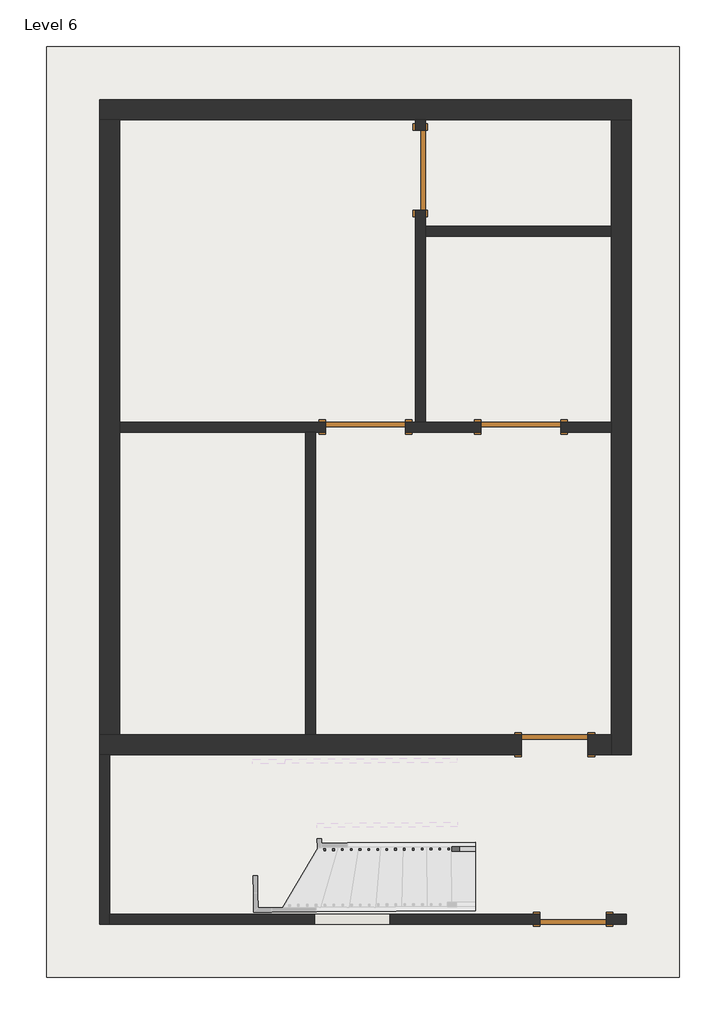
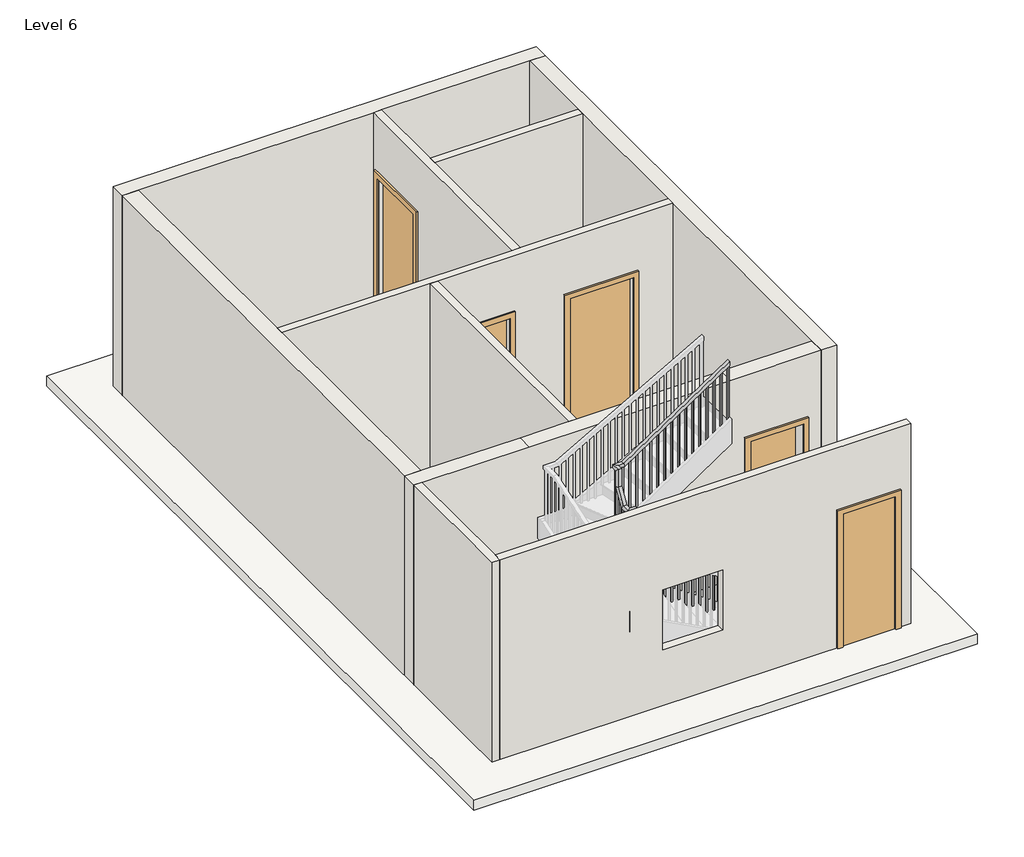
# One storey, part 1 of 2: 10 walls, 5 doors, 1 railing, 1 roof.
"""IFC4 building model written with IfcOpenShell, lengths in millimetres."""

from ifc_helpers import new_model, si_unit, frame, origin, place, context, project, spatial, polyline, outline, extrude, faceted_brep, transform, mapped, element, save
from components import door_a1484949, door_d8f5dbb5, door_e5f9f3c4, door_305aa2a5

model = new_model("IFC4")

# Units and contexts
model_context = context("Model", 3, world=origin())
ifc_project = project(units=[si_unit("LENGTHUNIT", "METRE", prefix="MILLI")], contexts=[model_context])

# Site, building, storey
site = spatial("IfcSite", under=ifc_project)
building = spatial("IfcBuilding", under=site)
storey = spatial("IfcBuildingStorey", under=building, Name="Level 6", Elevation=12801.6)

# Doors
placement = place(None, origin())
door_shape = door_a1484949(model_context)
element("IfcDoor", 1, ObjectType="Single-Flush : 30\" x 80\"", at=placement, inside=storey, context=model_context, shape_type="MappedRepresentation", body=[
    mapped(door_shape, transform((792.5410386, -2372.0109248, 12801.6), x_axis=(1.0, 0.0, 0.0), y_axis=(0.0, 1.0, 0.0), z_axis=(0.0, 0.0, 1.0))),
])
door_2_shape = door_d8f5dbb5(model_context)
element("IfcDoor", 2, ObjectType="Single-Flush : 30\" x 80\"", at=placement, inside=storey, context=model_context, shape_type="MappedRepresentation", body=[
    mapped(door_2_shape, transform((1002.0910386, -4372.2609248, 12801.6), x_axis=(-1.0, 0.0, 0.0), y_axis=(0.0, -1.0, 0.0), z_axis=(0.0, 0.0, 1.0))),
])
door_3_shape = door_e5f9f3c4(model_context)
element("IfcDoor", 3, ObjectType="Single-Flush : 36\" x 84\"", at=placement, inside=storey, context=model_context, shape_type="MappedRepresentation", body=[
    mapped(door_3_shape, transform((-750.5089614, 4209.7640752, 12801.6), x_axis=(0.0, -1.0, 0.0), y_axis=(1.0, 0.0, 0.0), z_axis=(0.0, 0.0, 1.0))),
])
door_4_shape = door_305aa2a5(model_context)
element("IfcDoor", 4, ObjectType="Single-Flush : 36\" x 84\"", at=placement, inside=storey, context=model_context, shape_type="MappedRepresentation", body=[
    mapped(door_4_shape, transform((402.0160386, 1266.5390752, 12801.6), x_axis=(-1.0, 0.0, 0.0), y_axis=(0.0, -1.0, 0.0), z_axis=(0.0, 0.0, 1.0))),
])
element("IfcDoor", 5, ObjectType="Single-Flush : 36\" x 84\"", at=placement, inside=storey, context=model_context, shape_type="MappedRepresentation", body=[
    mapped(door_4_shape, transform((-1379.1589614, 1266.5390752, 12801.6), x_axis=(-1.0, 0.0, 0.0), y_axis=(0.0, -1.0, 0.0), z_axis=(0.0, 0.0, 1.0))),
])

# Railing
element("IfcRailing", 6, ObjectType="Handrail - Rectangular", at=placement, inside=storey, context=model_context, shape_type="SolidModel", body=[
    faceted_brep([(-120.3816305, -3590.4209536, 13885.3333333), (-120.3816305, -3590.4209536, 13824.1630107), (-120.6930289, -3539.621908, 13824.1630107), (-120.6930289, -3539.621908, 13885.3333333), (-1854.5612186, -3601.0514854, 15048.6182998), (-1905.3602642, -3601.3628839, 15021.5238978), (-1905.6716627, -3550.5638383, 15021.5238978), (-1854.8726171, -3550.2524399, 15048.6182998), (-1854.5612186, -3601.0514854, 15270.8829276), (-1905.3602642, -3601.3628839, 15220.0829276), (-1905.6716627, -3550.5638383, 15220.0829276), (-1854.8726171, -3550.2524399, 15270.8829276), (-1981.5588325, -3601.8299816, 15270.8829276), (-1981.5588325, -3601.8299816, 15220.0829276), (-1931.0711854, -3550.7195376, 15220.0829276), (-1931.0711854, -3550.7195376, 15270.8829276), (-1982.3373287, -3474.8323677, 15270.8829276), (-1982.5128182, -3446.2044317, 15220.0829276), (-1931.7137726, -3445.8930332, 15220.0829276), (-1931.5382832, -3474.5209692, 15270.8829276), (-1983.1158249, -3347.8347538, 15480.6434812), (-1983.4272234, -3297.0357082, 15466.4632575), (-1932.6281778, -3296.7243097, 15466.4632575), (-1932.3167793, -3347.5233553, 15480.6434812), (-1983.1158249, -3347.8347538, 15752.0951436), (-1983.4272234, -3297.0357082, 15701.2951436), (-1932.6281778, -3296.7243097, 15701.2951436), (-1932.3167793, -3347.5233553, 15752.0951436), (-1983.8943211, -3220.8371398, 15752.0951436), (-1983.8943211, -3220.8371398, 15701.2951436), (-1932.783877, -3271.3247869, 15701.2951436), (-1932.783877, -3271.3247869, 15752.0951436), (-1856.8967072, -3220.0586437, 15752.0951436), (-1841.6341703, -3219.9650842, 15701.2951436), (-1841.3227719, -3270.7641298, 15701.2951436), (-1856.5853087, -3270.8576892, 15752.0951436), (-324.9523945, -3210.6678153, 16764.0), (-324.6409961, -3261.4668609, 16764.0), (-324.6409961, -3261.4668609, 16703.1185401), (-324.9523945, -3210.6678153, 16703.1185401)], [[[0, 1, 2, 3]], [[1, 0, 4, 5]], [[2, 1, 5, 6]], [[3, 2, 6, 7]], [[0, 3, 7, 4]], [[5, 4, 8, 9]], [[6, 5, 9, 10]], [[7, 6, 10, 11]], [[4, 7, 11, 8]], [[9, 8, 12, 13]], [[10, 9, 13, 14]], [[11, 10, 14, 15]], [[8, 11, 15, 12]], [[13, 12, 16, 17]], [[14, 13, 17, 18]], [[15, 14, 18, 19]], [[12, 15, 19, 16]], [[17, 16, 20, 21]], [[18, 17, 21, 22]], [[19, 18, 22, 23]], [[16, 19, 23, 20]], [[21, 20, 24, 25]], [[22, 21, 25, 26]], [[23, 22, 26, 27]], [[20, 23, 27, 24]], [[25, 24, 28, 29]], [[26, 25, 29, 30]], [[27, 26, 30, 31]], [[24, 27, 31, 28]], [[29, 28, 32, 33]], [[30, 29, 33, 34]], [[31, 30, 34, 35]], [[28, 31, 35, 32]], [[36, 37, 38, 39]], [[33, 32, 36, 39]], [[34, 33, 39, 38]], [[35, 34, 38, 37]], [[32, 35, 37, 36]]]),
    extrude(outline(polyline([(222.3085098, -19.05), (234.8914903, 0.0), (1246.1854534, 0.0), (1246.1854534, -19.05), (222.3085098, -19.05)])), frame((-342.2360746, -3245.6994205, 16926.4521201), z_axis=(-0.00612989118043648, 0.9999812120405643, 0.0), x_axis=(0.0, 0.0, -1.0)), (0.0, 0.0, 1.0), 19.05),
    extrude(outline(polyline([(222.3085098, -19.0499999), (234.8914902, 0.0), (1179.0762243, 0.0), (1179.0762243, -19.0499999), (222.3085098, -19.0499999)])), frame((-443.8341657, -3246.3222175, 16859.342891), z_axis=(-0.00612989118043648, 0.9999812120405643, 0.0), x_axis=(0.0, 0.0, -1.0)), (0.0, 0.0, 1.0), 19.05),
    extrude(outline(polyline([(222.3085098, -19.05), (234.8914902, 0.0), (1111.9669952, 0.0), (1111.9669952, -19.05), (222.3085098, -19.05)])), frame((-545.4322569, -3246.9450144, 16792.2336619), z_axis=(-0.00612989118043648, 0.9999812120405643, 0.0), x_axis=(0.0, 0.0, -1.0)), (0.0, 0.0, 1.0), 19.05),
    extrude(outline(polyline([(222.3085098, -19.05), (234.8914902, 0.0), (1214.1910995, 0.0), (1214.1910995, -19.05), (222.3085098, -19.05)])), frame((-647.030348, -3247.5678114, 16725.1244328), z_axis=(-0.00612989118043648, 0.9999812120405643, 0.0), x_axis=(0.0, 0.0, -1.0)), (0.0, 0.0, 1.0), 19.05),
    extrude(outline(polyline([(222.3085098, -19.05), (234.8914902, 0.0), (1147.0818704, 0.0), (1147.0818704, -19.05), (222.3085098, -19.05)])), frame((-748.6284392, -3248.1906083, 16658.0152037), z_axis=(-0.00612989118043648, 0.9999812120405643, 0.0), x_axis=(0.0, 0.0, -1.0)), (0.0, 0.0, 1.0), 19.05),
    extrude(outline(polyline([(222.3085098, -19.05), (234.8914902, 0.0), (1079.9726413, 0.0), (1079.9726413, -19.05), (222.3085098, -19.05)])), frame((-850.2265303, -3248.8134053, 16590.9059746), z_axis=(-0.00612989118043648, 0.9999812120405643, 0.0), x_axis=(0.0, 0.0, -1.0)), (0.0, 0.0, 1.0), 19.05),
    extrude(outline(polyline([(222.3085098, -19.05), (234.8914902, 0.0), (1182.1967455, 0.0), (1182.1967455, -19.05), (222.3085098, -19.05)])), frame((-951.8246215, -3249.4362022, 16523.7967455), z_axis=(-0.00612989118043648, 0.9999812120405643, 0.0), x_axis=(0.0, 0.0, -1.0)), (0.0, 0.0, 1.0), 19.05),
    extrude(outline(polyline([(222.3085097, -19.05), (234.8914902, 0.0), (1115.0875164, 0.0), (1115.0875164, -19.05), (222.3085097, -19.05)])), frame((-1053.4227126, -3250.0589992, 16456.6875164), z_axis=(-0.00612989118043648, 0.9999812120405643, 0.0), x_axis=(0.0, 0.0, -1.0)), (0.0, 0.0, 1.0), 19.05),
    extrude(outline(polyline([(222.3085097, -19.0499999), (234.8914902, 0.0), (1047.9782873, 0.0), (1047.9782873, -19.0499999), (222.3085097, -19.0499999)])), frame((-1155.0208037, -3250.6817961, 16389.5782873), z_axis=(-0.00612989118043648, 0.9999812120405643, 0.0), x_axis=(0.0, 0.0, -1.0)), (0.0, 0.0, 1.0), 19.05),
    extrude(outline(polyline([(222.3085097, -19.05), (234.8914902, 0.0), (1150.2023915, 0.0), (1150.2023915, -19.05), (222.3085097, -19.05)])), frame((-1256.6188949, -3251.304593, 16322.4690582), z_axis=(-0.00612989118043648, 0.9999812120405643, 0.0), x_axis=(0.0, 0.0, -1.0)), (0.0, 0.0, 1.0), 19.05),
    extrude(outline(polyline([(222.3085098, -19.05), (234.8914903, 0.0), (1083.0931625, 0.0), (1083.0931625, -19.05), (222.3085098, -19.05)])), frame((-1358.216986, -3251.92739, 16255.3598292), z_axis=(-0.00612989118043648, 0.9999812120405643, 0.0), x_axis=(0.0, 0.0, -1.0)), (0.0, 0.0, 1.0), 19.05),
    extrude(outline(polyline([(222.3085098, -19.05), (234.8914903, 0.0), (1185.3172668, 0.0), (1185.3172668, -19.05), (222.3085098, -19.05)])), frame((-1459.8150772, -3252.5501869, 16188.2506001), z_axis=(-0.00612989118043648, 0.9999812120405643, 0.0), x_axis=(0.0, 0.0, -1.0)), (0.0, 0.0, 1.0), 19.05),
    extrude(outline(polyline([(222.3085098, -19.05), (234.8914903, 0.0), (1118.2080377, 0.0), (1118.2080377, -19.05), (222.3085098, -19.05)])), frame((-1561.4131683, -3253.1729839, 16121.141371), z_axis=(-0.00612989118043648, 0.9999812120405643, 0.0), x_axis=(0.0, 0.0, -1.0)), (0.0, 0.0, 1.0), 19.05),
    extrude(outline(polyline([(222.3085098, -19.05), (234.8914902, 0.0), (1051.0988086, 0.0), (1051.0988086, -19.05), (222.3085098, -19.05)])), frame((-1663.0112595, -3253.7957808, 16054.0321419), z_axis=(-0.00612989118043648, 0.9999812120405643, 0.0), x_axis=(0.0, 0.0, -1.0)), (0.0, 0.0, 1.0), 19.05),
    extrude(outline(polyline([(222.3085098, -19.05), (234.8914902, 0.0), (1153.3229128, 0.0), (1153.3229128, -19.05), (222.3085098, -19.05)])), frame((-1764.6093506, -3254.4185778, 15986.9229128), z_axis=(-0.00612989118043648, 0.9999812120405643, 0.0), x_axis=(0.0, 0.0, -1.0)), (0.0, 0.0, 1.0), 19.05),
    extrude(outline(polyline([(222.3085098, -19.05), (234.8914902, 0.0), (1086.2136837, 0.0), (1086.2136837, -19.05), (222.3085098, -19.05)])), frame((-1866.2074418, -3255.0413747, 15919.8136837), z_axis=(-0.00612989118043648, 0.9999812120405643, 0.0), x_axis=(0.0, 0.0, -1.0)), (0.0, 0.0, 1.0), 19.05),
    extrude(outline(polyline([(-1948.6001916, -3280.94692), (-1967.6498337, -3281.0636944), (-1967.7666081, -3262.0140523), (-1948.716966, -3261.8972779), (-1948.6001916, -3280.94692)])), frame((0.0, 0.0, 14664.2666667), z_axis=(0.0, 0.0, 1.0), x_axis=(1.0, 0.0, 0.0)), (0.0, 0.0, 1.0), 1037.0284769),
    extrude(outline(polyline([(244.3320415, -19.05), (212.8679585, 0.0), (1074.2735921, 0.0), (1074.2735921, -19.05), (244.3320415, -19.05)])), frame((-1967.1438111, -3363.6121435, 15569.2069254), z_axis=(0.9999812120405644, 0.006129891180436036, 0.0), x_axis=(0.0, 0.0, -1.0)), (0.0, 0.0, 1.0), 19.05),
    extrude(outline(polyline([(244.3320415, -19.05), (212.8679585, 0.0), (1075.7984825, 0.0), (1075.7984825, -19.05), (244.3320415, -19.05)])), frame((-1966.5210142, -3465.2102346, 15401.3984825), z_axis=(0.9999812120405644, 0.006129891180436036, 0.0), x_axis=(0.0, 0.0, -1.0)), (0.0, 0.0, 1.0), 19.05),
    extrude(outline(polyline([(-1939.8365364, -3566.6485675), (-1939.719762, -3585.6982096), (-1958.7694041, -3585.814984), (-1958.8861785, -3566.7653419), (-1939.8365364, -3566.6485675)])), frame((0.0, 0.0, 14156.2666667), z_axis=(0.0, 0.0, 1.0), x_axis=(1.0, 0.0, 0.0)), (0.0, 0.0, 1.0), 1063.816261),
    extrude(outline(polyline([(234.9892351, -19.05), (222.2107648, 0.0), (1224.4109792, 0.0), (1224.4109792, -19.05), (234.9892351, -19.05)])), frame((-1857.171313, -3585.1921871, 15211.3443125), z_axis=(-0.006129891180436334, 0.9999812120405643, 0.0), x_axis=(0.0, 0.0, -1.0)), (0.0, 0.0, 1.0), 19.05),
    extrude(outline(polyline([(234.9892352, -19.05), (222.2107649, 0.0), (1156.259138, 0.0), (1156.259138, -19.05), (234.9892352, -19.05)])), frame((-1755.5732218, -3584.5693901, 15143.1924713), z_axis=(-0.006129891180436334, 0.9999812120405643, 0.0), x_axis=(0.0, 0.0, -1.0)), (0.0, 0.0, 1.0), 19.05),
    extrude(outline(polyline([(234.9892351, -19.05), (222.2107649, 0.0), (1257.44063, 0.0), (1257.44063, -19.05), (234.9892351, -19.05)])), frame((-1653.9751307, -3583.9465932, 15075.04063), z_axis=(-0.006129891180436334, 0.9999812120405643, 0.0), x_axis=(0.0, 0.0, -1.0)), (0.0, 0.0, 1.0), 19.05),
    extrude(outline(polyline([(234.9892351, -19.05), (222.2107649, 0.0), (1189.2887887, 0.0), (1189.2887887, -19.05), (234.9892351, -19.05)])), frame((-1552.3770395, -3583.3237962, 15006.8887887), z_axis=(-0.006129891180436334, 0.9999812120405643, 0.0), x_axis=(0.0, 0.0, -1.0)), (0.0, 0.0, 1.0), 19.05),
    extrude(outline(polyline([(234.9892351, -19.05), (222.2107649, 0.0), (1290.4702807, 0.0), (1290.4702807, -19.05), (234.9892351, -19.05)])), frame((-1450.7789484, -3582.7009993, 14938.7369474), z_axis=(-0.006129891180436334, 0.9999812120405643, 0.0), x_axis=(0.0, 0.0, -1.0)), (0.0, 0.0, 1.0), 19.05),
    extrude(outline(polyline([(234.9892351, -19.0499999), (222.2107649, 0.0), (1222.3184394, 0.0), (1222.3184394, -19.0499999), (234.9892351, -19.0499999)])), frame((-1349.1808572, -3582.0782024, 14870.5851061), z_axis=(-0.006129891180436334, 0.9999812120405643, 0.0), x_axis=(0.0, 0.0, -1.0)), (0.0, 0.0, 1.0), 19.05),
    extrude(outline(polyline([(234.9892351, -19.05), (222.2107648, 0.0), (1154.1665981, 0.0), (1154.1665981, -19.05), (234.9892351, -19.05)])), frame((-1247.5827661, -3581.4554054, 14802.4332648), z_axis=(-0.006129891180436334, 0.9999812120405643, 0.0), x_axis=(0.0, 0.0, -1.0)), (0.0, 0.0, 1.0), 19.05),
    extrude(outline(polyline([(234.9892352, -19.05), (222.2107649, 0.0), (1255.3480903, 0.0), (1255.3480903, -19.05), (234.9892352, -19.05)])), frame((-1145.984675, -3580.8326085, 14734.2814236), z_axis=(-0.006129891180436334, 0.9999812120405643, 0.0), x_axis=(0.0, 0.0, -1.0)), (0.0, 0.0, 1.0), 19.05),
    extrude(outline(polyline([(234.9892351, -19.05), (222.2107649, 0.0), (1187.196249, 0.0), (1187.196249, -19.05), (234.9892351, -19.05)])), frame((-1044.3865838, -3580.2098115, 14666.1295823), z_axis=(-0.006129891180436334, 0.9999812120405643, 0.0), x_axis=(0.0, 0.0, -1.0)), (0.0, 0.0, 1.0), 19.05),
    extrude(outline(polyline([(234.9892351, -19.05), (222.2107649, 0.0), (1288.377741, 0.0), (1288.377741, -19.05), (234.9892351, -19.05)])), frame((-942.7884927, -3579.5870146, 14597.977741), z_axis=(-0.006129891180436334, 0.9999812120405643, 0.0), x_axis=(0.0, 0.0, -1.0)), (0.0, 0.0, 1.0), 19.05),
    extrude(outline(polyline([(234.9892351, -19.05), (222.2107649, 0.0), (1220.2258997, 0.0), (1220.2258997, -19.05), (234.9892351, -19.05)])), frame((-841.1904015, -3578.9642176, 14529.8258997), z_axis=(-0.006129891180436334, 0.9999812120405643, 0.0), x_axis=(0.0, 0.0, -1.0)), (0.0, 0.0, 1.0), 19.05),
    extrude(outline(polyline([(234.9892351, -19.05), (222.2107649, 0.0), (1152.0740584, 0.0), (1152.0740584, -19.05), (234.9892351, -19.05)])), frame((-739.5923104, -3578.3414207, 14461.6740584), z_axis=(-0.006129891180436334, 0.9999812120405643, 0.0), x_axis=(0.0, 0.0, -1.0)), (0.0, 0.0, 1.0), 19.05),
    extrude(outline(polyline([(234.9892351, -19.0499999), (222.2107648, 0.0), (1253.2555504, 0.0), (1253.2555504, -19.0499999), (234.9892351, -19.0499999)])), frame((-637.9942192, -3577.7186237, 14393.5222171), z_axis=(-0.006129891180436334, 0.9999812120405643, 0.0), x_axis=(0.0, 0.0, -1.0)), (0.0, 0.0, 1.0), 19.05),
    extrude(outline(polyline([(234.9892352, -19.05), (222.2107649, 0.0), (1185.1037092, 0.0), (1185.1037092, -19.05), (234.9892352, -19.05)])), frame((-536.3961281, -3577.0958268, 14325.3703759), z_axis=(-0.006129891180436334, 0.9999812120405643, 0.0), x_axis=(0.0, 0.0, -1.0)), (0.0, 0.0, 1.0), 19.05),
    extrude(outline(polyline([(234.9892351, -19.05), (222.2107649, 0.0), (1116.9518679, 0.0), (1116.9518679, -19.05), (234.9892351, -19.05)])), frame((-434.798037, -3576.4730299, 14257.2185346), z_axis=(-0.006129891180436334, 0.9999812120405643, 0.0), x_axis=(0.0, 0.0, -1.0)), (0.0, 0.0, 1.0), 19.05),
    extrude(outline(polyline([(234.9892351, -19.05), (222.2107649, 0.0), (1218.13336, 0.0), (1218.13336, -19.05), (234.9892351, -19.05)])), frame((-333.1999458, -3575.8502329, 14189.0666933), z_axis=(-0.006129891180436334, 0.9999812120405643, 0.0), x_axis=(0.0, 0.0, -1.0)), (0.0, 0.0, 1.0), 19.05),
    extrude(outline(polyline([(234.9892351, -19.05), (222.2107649, 0.0), (1149.9815187, 0.0), (1149.9815187, -19.05), (234.9892351, -19.05)])), frame((-231.6018547, -3575.227436, 14120.914852), z_axis=(-0.006129891180436334, 0.9999812120405643, 0.0), x_axis=(0.0, 0.0, -1.0)), (0.0, 0.0, 1.0), 19.05),
    extrude(outline(polyline([(-1948.7558908, -3255.5473972), (-1967.8055329, -3255.6641716), (-1967.9223073, -3236.6145296), (-1948.8726652, -3236.4977551), (-1948.7558908, -3255.5473972)])), frame((0.0, 0.0, 14664.2666667), z_axis=(0.0, 0.0, 1.0), x_axis=(1.0, 0.0, 0.0)), (0.0, 0.0, 1.0), 1037.0284769),
    extrude(outline(polyline([(-1946.8485752, -3566.6915513), (-1946.7318007, -3585.7411934), (-1965.7814428, -3585.8579679), (-1965.8982173, -3566.8083258), (-1946.8485752, -3566.6915513)])), frame((0.0, 0.0, 14156.2666667), z_axis=(0.0, 0.0, 1.0), x_axis=(1.0, 0.0, 0.0)), (0.0, 0.0, 1.0), 1063.816261),
    extrude(outline(polyline([(222.3085098, -19.05), (234.8914902, 0.0), (1245.1603832, 0.0), (1245.1603832, -19.05), (222.3085098, -19.05)])), frame((-343.7879502, -3245.7089335, 16925.4270499), z_axis=(-0.00612989118043648, 0.9999812120405643, 0.0), x_axis=(0.0, 0.0, -1.0)), (0.0, 0.0, 1.0), 19.05),
    extrude(outline(polyline([(234.9892351, -19.05), (222.2107648, 0.0), (1088.2189125, 0.0), (1088.2189125, -19.05), (234.9892351, -19.05)])), frame((-139.5285846, -3574.6630262, 14059.1522458), z_axis=(-0.006129891180436334, 0.9999812120405643, 0.0), x_axis=(0.0, 0.0, -1.0)), (0.0, 0.0, 1.0), 19.05),
])

# Roof
element("IfcRoof", 7, ObjectType="Generic - 12\"", at=placement, inside=storey, context=model_context, shape_type="SweptSolid", body=[
    extrude(outline(polyline([(-5036.7589614, 5628.9890752), (2221.2910386, 5628.9890752), (2221.2910386, -5039.0109248), (-5036.7589614, -5039.0109248), (-5036.7589614, 5628.9890752)])), frame((0.0, 0.0, 12649.2), z_axis=(0.0, 0.0, 1.0), x_axis=(1.0, 0.0, 0.0)), (0.0, 0.0, 1.0), 152.4),
])

# Walls
element("IfcWall", 8, ObjectType="4.5\"", at=placement, inside=storey, context=model_context, shape_type="Brep", body=[
    faceted_brep([(-807.6589614, 3752.5640752, 14935.2), (-807.6589614, 3752.5640752, 12801.6), (-807.6589614, 1323.6890752, 12801.6), (-807.6589614, 1323.6890752, 15849.6), (-807.6589614, 4790.7890752, 15849.6), (-807.6589614, 4790.7890752, 12801.6), (-807.6589614, 4666.9640752, 12801.6), (-807.6589614, 4666.9640752, 14935.2), (-693.3589614, 1323.6890752, 12801.6), (-693.3589614, 3457.2890752, 12801.6), (-693.3589614, 3571.5890752, 12801.6), (-693.3589614, 3752.5640752, 12801.6), (-693.3589614, 3752.5640752, 14935.2), (-693.3589614, 4666.9640752, 14935.2), (-693.3589614, 4666.9640752, 12801.6), (-693.3589614, 4790.7890752, 12801.6), (-693.3589614, 4790.7890752, 15849.6), (-693.3589614, 3571.5890752, 15849.6), (-693.3589614, 3457.2890752, 15849.6), (-693.3589614, 1323.6890752, 15849.6)], [[[0, 1, 2, 3, 4, 5, 6, 7]], [[8, 9, 10, 11, 12, 13, 14, 15, 16, 17, 18, 19]], [[6, 5, 15, 14]], [[2, 1, 11, 10, 9, 8]], [[5, 4, 16, 15]], [[3, 2, 8, 19]], [[12, 11, 1, 0]], [[13, 12, 0, 7]], [[14, 13, 7, 6]], [[4, 3, 19, 18, 17, 16]]]),
])
element("IfcWall", 9, ObjectType="4.5\"", at=placement, inside=storey, context=model_context, shape_type="SweptSolid", body=[
    extrude(outline(polyline([(-693.3589614, 3571.5890752), (1440.2410386, 3571.5890752), (1440.2410386, 3457.2890752), (-693.3589614, 3457.2890752), (-693.3589614, 3571.5890752)])), frame((0.0, 0.0, 12801.6), z_axis=(0.0, 0.0, 1.0), x_axis=(1.0, 0.0, 0.0)), (0.0, 0.0, 1.0), 3048.0),
])
element("IfcWall", 10, ObjectType="4.5\"", at=placement, inside=storey, context=model_context, shape_type="Brep", body=[
    faceted_brep([(-4198.5589614, 1209.3890752, 12801.6), (-2064.9589614, 1209.3890752, 12801.6), (-1950.6589614, 1209.3890752, 12801.6), (-1836.3589614, 1209.3890752, 12801.6), (-1836.3589614, 1209.3890752, 14935.2), (-921.9589614, 1209.3890752, 14935.2), (-921.9589614, 1209.3890752, 12801.6), (-55.1839614, 1209.3890752, 12801.6), (-55.1839614, 1209.3890752, 14935.2), (859.2160386, 1209.3890752, 14935.2), (859.2160386, 1209.3890752, 12801.6), (1440.2410386, 1209.3890752, 12801.6), (1440.2410386, 1209.3890752, 15849.6), (-1950.6589614, 1209.3890752, 15849.6), (-2064.9589614, 1209.3890752, 15849.6), (-4198.5589614, 1209.3890752, 15849.6), (-1836.3589614, 1323.6890752, 14935.2), (-1836.3589614, 1323.6890752, 12801.6), (-4198.5589614, 1323.6890752, 12801.6), (-4198.5589614, 1323.6890752, 15849.6), (-807.6589614, 1323.6890752, 15849.6), (-693.3589614, 1323.6890752, 15849.6), (1440.2410386, 1323.6890752, 15849.6), (1440.2410386, 1323.6890752, 12801.6), (859.2160386, 1323.6890752, 12801.6), (859.2160386, 1323.6890752, 14935.2), (-55.1839614, 1323.6890752, 14935.2), (-55.1839614, 1323.6890752, 12801.6), (-693.3589614, 1323.6890752, 12801.6), (-807.6589614, 1323.6890752, 12801.6), (-921.9589614, 1323.6890752, 12801.6), (-921.9589614, 1323.6890752, 14935.2)], [[[0, 1, 2, 3, 4, 5, 6, 7, 8, 9, 10, 11, 12, 13, 14, 15]], [[16, 17, 18, 19, 20, 21, 22, 23, 24, 25, 26, 27, 28, 29, 30, 31]], [[24, 23, 11, 10]], [[18, 17, 3, 2, 1, 0]], [[30, 29, 28, 27, 7, 6]], [[12, 11, 23, 22]], [[0, 15, 19, 18]], [[8, 7, 27, 26]], [[9, 8, 26, 25]], [[10, 9, 25, 24]], [[4, 3, 17, 16]], [[5, 4, 16, 31]], [[6, 5, 31, 30]], [[15, 14, 13, 12, 22, 21, 20, 19]]]),
])
element("IfcWall", 11, ObjectType="4.5\"", at=placement, inside=storey, context=model_context, shape_type="SweptSolid", body=[
    extrude(outline(polyline([(-2064.9589614, -2257.7109248), (-2064.9589614, 1209.3890752), (-1950.6589614, 1209.3890752), (-1950.6589614, -2257.7109248), (-2064.9589614, -2257.7109248)])), frame((0.0, 0.0, 12801.6), z_axis=(0.0, 0.0, 1.0), x_axis=(1.0, 0.0, 0.0)), (0.0, 0.0, 1.0), 3048.0),
])
element("IfcWall", 12, ObjectType="4.5\"", at=placement, inside=storey, context=model_context, shape_type="Brep", body=[
    faceted_brep([(-4427.1589614, -2486.3109248, 12801.6), (-4427.1589614, -4429.4109248, 12801.6), (-4427.1589614, -4429.4109248, 15849.6), (-4427.1589614, -2486.3109248, 15849.6), (-4312.8589614, -2486.3109248, 12801.6), (-4312.8589614, -2486.3109248, 15849.6), (-4312.8589614, -4315.1109248, 15849.6), (-4312.8589614, -4429.4109248, 15849.6), (-4312.8589614, -4429.4109248, 12801.6), (-4312.8589614, -4315.1109248, 12801.6)], [[[0, 1, 2, 3]], [[4, 5, 6, 7, 8, 9]], [[1, 0, 4, 9, 8]], [[3, 2, 7, 6, 5]], [[0, 3, 5, 4]], [[2, 1, 8, 7]]]),
])
element("IfcWall", 13, ObjectType="4.5\"", at=placement, inside=storey, context=model_context, shape_type="SweptSolid", body=[
    extrude(outline(polyline([(12801.6, -4312.8589614), (12801.6, 621.0910386), (14833.6, 621.0910386), (14833.6, 1383.0910386), (12801.6, 1383.0910386), (12801.6, 1611.6910386), (15849.6, 1611.6910386), (15849.6, -4312.8589614), (12801.6, -4312.8589614)]), holes=[polyline([(14569.3567311, -1963.3589614), (14569.3567311, -1099.7589614), (13654.9567311, -1099.7589614), (13654.9567311, -1963.3589614), (14569.3567311, -1963.3589614)])]), frame((0.0, -4429.4109248, 0.0), z_axis=(0.0, 1.0, 0.0), x_axis=(0.0, 0.0, 1.0)), (0.0, 0.0, 1.0), 114.3),
])
element("IfcWall", 14, ObjectType="9\"", at=placement, inside=storey, context=model_context, shape_type="Brep", body=[
    faceted_brep([(-4427.1589614, 4790.7890752, 12801.6), (-4198.5589614, 4790.7890752, 12801.6), (-807.6589614, 4790.7890752, 12801.6), (-693.3589614, 4790.7890752, 12801.6), (1440.2410386, 4790.7890752, 12801.6), (1668.8410386, 4790.7890752, 12801.6), (1668.8410386, 4790.7890752, 15849.6), (1440.2410386, 4790.7890752, 15849.6), (-693.3589614, 4790.7890752, 15849.6), (-807.6589614, 4790.7890752, 15849.6), (-4198.5589614, 4790.7890752, 15849.6), (-4427.1589614, 4790.7890752, 15849.6), (-4427.1589614, 5019.3890752, 12801.6), (-4427.1589614, 5019.3890752, 15849.6), (1668.8410386, 5019.3890752, 15849.6), (1668.8410386, 5019.3890752, 12801.6)], [[[0, 1, 2, 3, 4, 5, 6, 7, 8, 9, 10, 11]], [[12, 13, 14, 15]], [[5, 4, 3, 2, 1, 0, 12, 15]], [[6, 5, 15, 14]], [[0, 11, 13, 12]], [[11, 10, 9, 8, 7, 6, 14, 13]]]),
])
element("IfcWall", 15, ObjectType="9\"", at=placement, inside=storey, context=model_context, shape_type="Brep", body=[
    faceted_brep([(1440.2410386, 4790.7890752, 12801.6), (1440.2410386, 3571.5890752, 12801.6), (1440.2410386, 3457.2890752, 12801.6), (1440.2410386, 1323.6890752, 12801.6), (1440.2410386, 1209.3890752, 12801.6), (1440.2410386, -2257.7109248, 12801.6), (1440.2410386, -2486.3109248, 12801.6), (1440.2410386, -2486.3109248, 15849.6), (1440.2410386, -2257.7109248, 15849.6), (1440.2410386, 1209.3890752, 15849.6), (1440.2410386, 1323.6890752, 15849.6), (1440.2410386, 3457.2890752, 15849.6), (1440.2410386, 3571.5890752, 15849.6), (1440.2410386, 4790.7890752, 15849.6), (1668.8410386, 4790.7890752, 12801.6), (1668.8410386, 4790.7890752, 15849.6), (1668.8410386, -2486.3109248, 15849.6), (1668.8410386, -2486.3109248, 12801.6)], [[[0, 1, 2, 3, 4, 5, 6, 7, 8, 9, 10, 11, 12, 13]], [[14, 15, 16, 17]], [[6, 5, 4, 3, 2, 1, 0, 14, 17]], [[0, 13, 15, 14]], [[7, 6, 17, 16]], [[13, 12, 11, 10, 9, 8, 7, 16, 15]]]),
])
element("IfcWall", 16, ObjectType="9\"", at=placement, inside=storey, context=model_context, shape_type="Brep", body=[
    faceted_brep([(1440.2410386, -2257.7109248, 12801.6), (1173.5410386, -2257.7109248, 12801.6), (1173.5410386, -2257.7109248, 14833.6), (411.5410386, -2257.7109248, 14833.6), (411.5410386, -2257.7109248, 12801.6), (-1950.6589614, -2257.7109248, 12801.6), (-2064.9589614, -2257.7109248, 12801.6), (-4198.5589614, -2257.7109248, 12801.6), (-4427.1589614, -2257.7109248, 12801.6), (-4427.1589614, -2257.7109248, 15849.6), (-4198.5589614, -2257.7109248, 15849.6), (-2764.4103136, -2257.7109248, 15849.6), (-2064.9589614, -2257.7109248, 15849.6), (-1950.6589614, -2257.7109248, 15849.6), (131.1896864, -2257.7109248, 15849.6), (1440.2410386, -2257.7109248, 15849.6), (1173.5410386, -2486.3109248, 14833.6), (1173.5410386, -2486.3109248, 12801.6), (1440.2410386, -2486.3109248, 12801.6), (1440.2410386, -2486.3109248, 15849.6), (131.1896864, -2486.3109248, 15849.6), (-2764.4103136, -2486.3109248, 15849.6), (-4312.8589614, -2486.3109248, 15849.6), (-4427.1589614, -2486.3109248, 15849.6), (-4427.1589614, -2486.3109248, 12801.6), (-4312.8589614, -2486.3109248, 12801.6), (411.5410386, -2486.3109248, 12801.6), (411.5410386, -2486.3109248, 14833.6), (-2764.4103136, -2269.417212, 15849.6), (131.1896864, -2269.417212, 15849.6)], [[[0, 1, 2, 3, 4, 5, 6, 7, 8, 9, 10, 11, 12, 13, 14, 15]], [[16, 17, 18, 19, 20, 21, 22, 23, 24, 25, 26, 27]], [[18, 17, 1, 0]], [[26, 25, 24, 8, 7, 6, 5, 4]], [[0, 15, 19, 18]], [[9, 8, 24, 23]], [[2, 1, 17, 16]], [[3, 2, 16, 27]], [[4, 3, 27, 26]], [[14, 13, 12, 11, 28, 21, 20, 29]], [[11, 10, 9, 23, 22, 21, 28]], [[15, 14, 29, 20, 19]]]),
])
element("IfcWall", 17, ObjectType="9\"", at=placement, inside=storey, context=model_context, shape_type="Brep", body=[
    faceted_brep([(-4198.5589614, -2257.7109248, 12801.6), (-4198.5589614, 1209.3890752, 12801.6), (-4198.5589614, 1323.6890752, 12801.6), (-4198.5589614, 4790.7890752, 12801.6), (-4198.5589614, 4790.7890752, 15849.6), (-4198.5589614, 1323.6890752, 15849.6), (-4198.5589614, 1209.3890752, 15849.6), (-4198.5589614, -2257.7109248, 15849.6), (-4427.1589614, -2257.7109248, 12801.6), (-4427.1589614, -2257.7109248, 15849.6), (-4427.1589614, 4790.7890752, 15849.6), (-4427.1589614, 4790.7890752, 12801.6)], [[[0, 1, 2, 3, 4, 5, 6, 7]], [[8, 9, 10, 11]], [[3, 2, 1, 0, 8, 11]], [[0, 7, 9, 8]], [[4, 3, 11, 10]], [[7, 6, 5, 4, 10, 9]]]),
])

save(model, "model.ifc")

# Revit data of these elements
# Type "Single-Flush : 30\" x 80\""
#   Type Mark = "5"
#   Construction Type Id = "MDOOR"
#   Assembly Code = "C1020"
#   Analytic Construction = "Metal"
#   Thickness = 0' - 2"
#   Heat Transfer Coefficient (U) = 0.651978 BTU/(h·ft²·°F)
#   Height = 6' - 8"
#   Trim Projection Ext = 0' - 1"
#   Trim Projection Int = 0' - 1"
#   Trim Width = 0' - 3"
#   Width = 2' - 6"
#   Define Thermal Properties by = 1
#   Define Thermal Properties by = 1
#   Door Material = Door - Panel
#   Frame Material = Door - Frame
#   Visual Light Transmittance = 0
#   Solar Heat Gain Coefficient = 0
#   Function = (empty or 0)
#   Wall Closure = (empty or 0)
# Type "Single-Flush : 36\" x 84\""
#   Type Mark = "1"
#   Construction Type Id = "MDOOR"
#   Assembly Code = "C1020"
#   Analytic Construction = "Metal"
#   Thickness = 0' - 2"
#   Heat Transfer Coefficient (U) = 0.651978 BTU/(h·ft²·°F)
#   Height = 7' - 0"
#   Trim Projection Ext = 0' - 1"
#   Trim Projection Int = 0' - 1"
#   Trim Width = 0' - 3"
#   Width = 3' - 0"
#   Define Thermal Properties by = 1
#   Define Thermal Properties by = 1
#   Door Material = Door - Panel
#   Frame Material = Door - Frame
#   Visual Light Transmittance = 0
#   Solar Heat Gain Coefficient = 0
#   Function = (empty or 0)
#   Wall Closure = (empty or 0)
# Type "Handrail - Rectangular"
#   Assembly Code = "C2010400"
#   built-in parameter 1008612 = 0.0416667 (stored number, unit not read)
#   built-in parameter 1008611 = 0.0416667 (stored number, unit not read)
#   built-in parameter 1008609 = 0.333333 (stored number, unit not read)
#   built-in parameter 1008604 = 0.166667 (stored number, unit not read)
#   built-in parameter 1008603 = 0.166667 (stored number, unit not read)
#   Railing Height = 3' - 0"
#   built-in parameter 1008630 = 2
#   built-in parameter 1008610 = 2
#   built-in parameter 1008618 = Baluster - Square : 3/4"
# Type "Generic - 12\""
#   Assembly Code = "B1020"
#   Layers, outside or top first: 0' - 6" no material (function 1)
# Type "4.5\""
#   Assembly Code = "B2010"
#   Layers, outside or top first: 0' - 4 1/2" no material (function 1)
# Type "9\""
#   Assembly Code = "B2010"
#   Layers, outside or top first: 0' - 9" no material (function 1)
# Elements 1, 2 (IfcDoor, "Single-Flush : 30\" x 80\"")
#   Phase Created = New Construction
#   Materials on its faces: "Door - Frame", "Door - Panel"
# Elements 3, 4, 5 (IfcDoor, "Single-Flush : 36\" x 84\"")
#   Phase Created = New Construction
#   Materials on its faces: "Door - Frame", "Door - Panel"
# Element 6 (IfcRailing, "Handrail - Rectangular")
#   Phase Created = New Construction
# Element 7 (IfcRoof, "Generic - 12\"")
#   built-in parameter 1001705 = 42 (stored number, unit not read)
#   built-in parameter 1001701 = -0.5 (stored number, unit not read)
#   built-in parameter 1001710 = 33615
#   Phase Created = New Construction
#   Materials on its faces: "Default Roof", "Door - Frame"
# Elements 8, 9, 10, 11 (IfcWall, "4.5\"")
#   Top Offset = 0' - 0"
#   Base Offset = 0' - 0"
#   Unconnected Height = 10' - 0"
#   wall height = 10' - 0"
#   Phase Created = New Construction
#   Base Constraint = Level 6
#   Materials on its faces: "Default Wall"
# Elements 12, 13 (IfcWall, "4.5\"")
#   Top Offset = 0' - 0"
#   Base Offset = 0' - 0"
#   Unconnected Height = 10' - 0"
#   wall height = 10' - 0"
#   Phase Created = New Construction
#   Base Constraint = Level 6
#   Materials on its faces: "Default Wall", "Door - Frame"
# Elements 14, 15, 16, 17 (IfcWall, "9\"")
#   Top Offset = 0' - 0"
#   Base Offset = 0' - 0"
#   Unconnected Height = 10' - 0"
#   wall height = 10' - 0"
#   Phase Created = New Construction
#   Base Constraint = Level 6
#   Materials on its faces: "Default Wall", "Door - Frame"
# Materials
#   "Door - Panel": class "Wood", colour RGB 210 159 95, transparency 0, Cost = 0
#   "Door - Frame": colour RGB 118 70 51, transparency 0, Cost = 0
#   "Default Roof": colour RGB 88 101 114, transparency 0, Cost = 0
#   "Default Wall": colour RGB 128 128 128, transparency 0, Cost = 0
